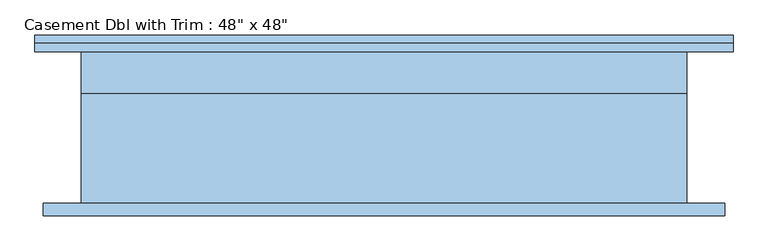
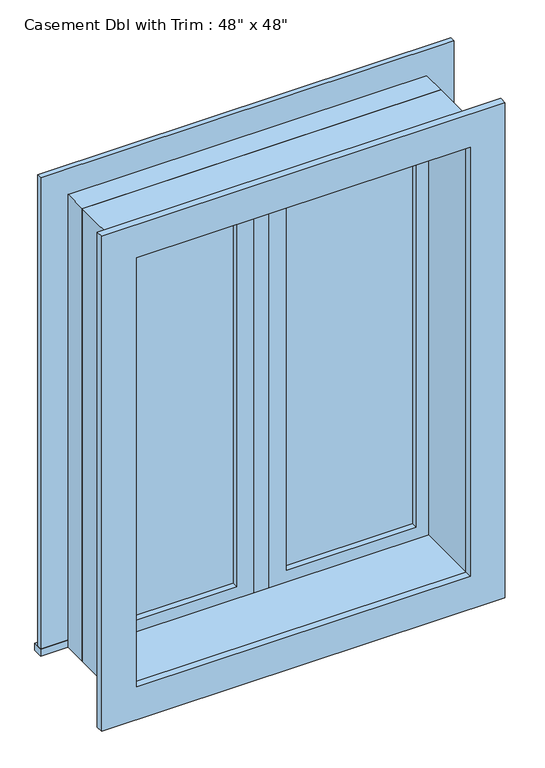
"""IFC4 building model written with IfcOpenShell, lengths in millimetres: window geometry."""

from ifc_helpers import new_model, si_unit, frame, origin, place, context, project, spatial, polyline, outline, extrude, source, transform, mapped, element, save


def window_419b5846(model_context):
    return source(origin(), model_context, "Body", "SweptSolid", [
        extrude(outline(polyline([(63.5, 98.425), (393.7, 98.425), (393.7, 85.725), (63.5, 85.725), (63.5, 98.425)])), frame((0.0, 0.0, 977.9), z_axis=(0.0, 0.0, 1.0), x_axis=(1.0, 0.0, 0.0)), (0.0, 0.0, 1.0), 1092.2),
        extrude(outline(polyline([(2114.55, 19.05), (933.45, 19.05), (933.45, 438.15), (2114.55, 438.15), (2114.55, 19.05)]), holes=[polyline([(2070.1, 63.5), (2070.1, 393.7), (977.9, 393.7), (977.9, 63.5), (2070.1, 63.5)])]), frame((0.0, 69.85, 0.0), z_axis=(0.0, 1.0, 0.0), x_axis=(0.0, 0.0, 1.0)), (0.0, 0.0, 1.0), 44.45),
        extrude(outline(polyline([(19.05, 69.85), (-19.05, 69.85), (-19.05, 133.35), (19.05, 133.35), (19.05, 69.85)])), frame((0.0, 0.0, 933.45), z_axis=(0.0, 0.0, 1.0), x_axis=(1.0, 0.0, 0.0)), (0.0, 0.0, 1.0), 1181.1),
        extrude(outline(polyline([(-527.05, 158.75), (527.05, 158.75), (527.05, 133.35), (-527.05, 133.35), (-527.05, 158.75)])), frame((0.0, 0.0, 914.4), z_axis=(0.0, 0.0, 1.0), x_axis=(1.0, 0.0, 0.0)), (0.0, 0.0, 1.0), 19.05),
        extrude(outline(polyline([(2114.55, -438.15), (2114.55, 438.15), (933.45, 438.15), (933.45, 527.05), (2203.45, 527.05), (2203.45, -527.05), (933.45, -527.05), (933.45, -438.15), (2114.55, -438.15)])), frame((0.0, 133.35, 0.0), z_axis=(0.0, 1.0, 0.0), x_axis=(0.0, 0.0, 1.0)), (0.0, 0.0, 1.0), 12.7),
        extrude(outline(polyline([(2190.75, 514.35), (2190.75, -514.35), (857.25, -514.35), (857.25, 514.35), (2190.75, 514.35)]), holes=[polyline([(2101.85, 425.45), (946.15, 425.45), (946.15, -425.45), (2101.85, -425.45), (2101.85, 425.45)])]), frame((0.0, -114.3, 0.0), z_axis=(0.0, 1.0, 0.0), x_axis=(0.0, 0.0, 1.0)), (0.0, 0.0, 1.0), 19.05),
        extrude(outline(polyline([(-63.5, 85.725), (-393.7, 85.725), (-393.7, 98.425), (-63.5, 98.425), (-63.5, 85.725)])), frame((0.0, 0.0, 977.9), z_axis=(0.0, 0.0, 1.0), x_axis=(1.0, 0.0, 0.0)), (0.0, 0.0, 1.0), 1092.2),
        extrude(outline(polyline([(2114.55, -438.15), (933.45, -438.15), (933.45, -19.05), (2114.55, -19.05), (2114.55, -438.15)]), holes=[polyline([(2070.1, -393.7), (2070.1, -63.5), (977.9, -63.5), (977.9, -393.7), (2070.1, -393.7)])]), frame((0.0, 69.85, 0.0), z_axis=(0.0, 1.0, 0.0), x_axis=(0.0, 0.0, 1.0)), (0.0, 0.0, 1.0), 44.45),
        extrude(outline(polyline([(2133.6, -457.2), (914.4, -457.2), (914.4, 457.2), (2133.6, 457.2), (2133.6, -457.2)]), holes=[polyline([(2101.85, -425.45), (2101.85, 425.45), (946.15, 425.45), (946.15, -425.45), (2101.85, -425.45)])]), frame((0.0, -95.25, 0.0), z_axis=(0.0, 1.0, 0.0), x_axis=(0.0, 0.0, 1.0)), (0.0, 0.0, 1.0), 165.1),
        extrude(outline(polyline([(2133.6, 457.2), (2133.6, -457.2), (914.4, -457.2), (914.4, 457.2), (2133.6, 457.2)]), holes=[polyline([(2114.55, 438.15), (933.45, 438.15), (933.45, -438.15), (2114.55, -438.15), (2114.55, 438.15)])]), frame((0.0, 69.85, 0.0), z_axis=(0.0, 1.0, 0.0), x_axis=(0.0, 0.0, 1.0)), (0.0, 0.0, 1.0), 63.5),
    ])


if __name__ == "__main__":
    model = new_model("IFC4")
    model_context = context("Model", 3, world=origin())
    ifc_project = project(units=[si_unit("LENGTHUNIT", "METRE", prefix="MILLI")], contexts=[model_context])
    site = spatial("IfcSite", under=ifc_project)
    building = spatial("IfcBuilding", under=site)
    placement = place(None, origin())
    window_shape = window_419b5846(model_context)
    element("IfcWindow", 1, ObjectType="Casement Dbl with Trim : 48\" x 48\"", at=placement, inside=building, context=model_context, shape_type="MappedRepresentation", body=[
        mapped(window_shape, transform((0.0, 0.0, 0.0), x_axis=(1.0, 0.0, 0.0), y_axis=(0.0, 1.0, 0.0), z_axis=(0.0, 0.0, 1.0))),
    ])
    save(model, "model.ifc")

# Revit data of these elements
# Type "Casement Dbl with Trim : 48\" x 48\""
#   Type Mark = "10"
#   Construction Type Id = "GSP4R"
#   Assembly Code = "B2020100"
#   Analytic Construction = "1/8 in Pilkington single glazing"
#   Visual Light Transmittance = 0.9
#   Solar Heat Gain Coefficient = 0.78
#   Heat Transfer Coefficient (U) = 0.6496 BTU/(h·ft²·°F)
#   Height = 4' - 0"
#   Default Sill Height = 3' - 0"
#   Trim Projection - Ext. = 0' - 0 1/2"
#   Trim Projection - Int. = 0' - 0 3/4"
#   Trim Width - Exterior = 0' - 3 1/2"
#   Trim Width - Interior = 0' - 3 1/2"
#   Width = 3' - 0"
#   Window Inset = 0' - 0 3/4"
#   Define Thermal Properties by = 1
#   Glass Pane Material = Glass
#   Sash Material = Sash
#   Trim Exterior Material = Trim
#   Trim Interior Material = Trim
#   Wall Closure = (empty or 0)
# Element 1 (IfcWindow, "Casement Dbl with Trim : 48\" x 48\"")
#   Materials on its faces: "Sash", "Trim", "Glass"
# Materials
#   "Glass": class "Glass", colour RGB 0 128 192, transparency 0.75, Description = "Soda Lime Glass", Cost = 0
#   "Sash": class "Wood", colour RGB 224 178 126, transparency 0
#   "Trim": class "Wood", colour RGB 224 178 126, transparency 0
